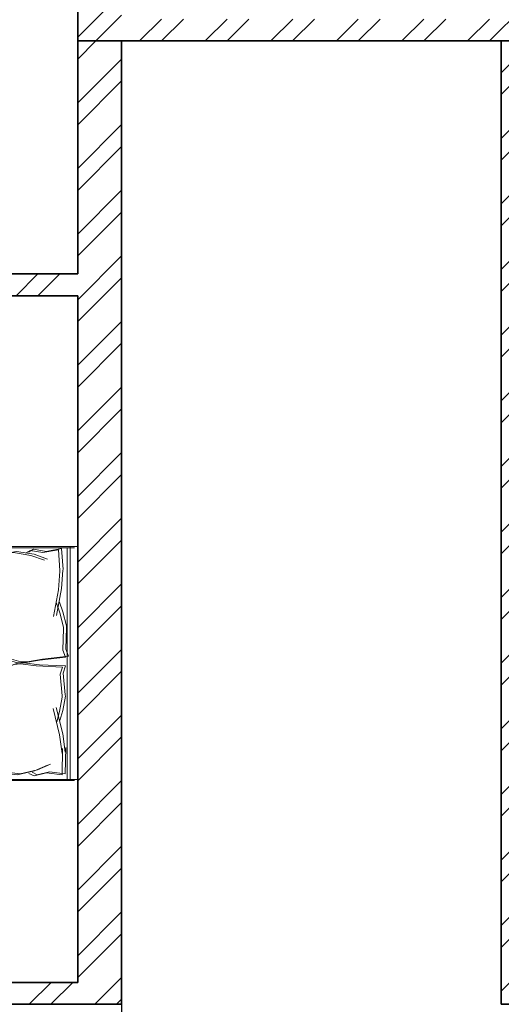
# Model space of a CAD drawing. Units: inches. Extents: x 2120 to 4013, y 1390 to 3019.
# Tile 13 of 59: x 2617 to 2716, y 1582 to 1784. Entities that reach past the tile are written whole.
import ezdxf

# ---------------------------------------------------------------- set-up
doc = ezdxf.new("R2010")
doc.units = ezdxf.units.IN
for name, color, linetype, lineweight in [('A-FLOR-DECK', 7, 'Continuous', 25), ('A-FURN', 8, 'Continuous', 13), ('A-WALL', 7, 'Continuous', 35), ('A-WALL-PATT', 252, 'Continuous', 13)]:
    doc.layers.add(name, color=color, linetype=linetype, lineweight=lineweight)

# ---------------------------------------------------------------- blocks, each defined once
blk = doc.blocks.new('BED-DOUBLE-PLAN')
for p, q in [((3.48, 63.34), (3.48, 81.45)), ((3.48, 81.45), (51.27, 81.45)), ((51.27, 81.45), (51.27, 54.84)), ((3.48, 79.91), (51.27, 79.91)), ((3.7, 62.7), (3.7, 80.81)), ((3.7, 79.27), (51.5, 79.27)), ((16.88, 78.42), (19.77, 79.14)), ((19.77, 79.14), (20.09, 79.14)), ((20.09, 79.14), (24.54, 79)), ((24.54, 79), (25.98, 79.58)), ((24.77, 78.36), (26.21, 78.94)), ((25.98, 79.58), (26.56, 74.23)), ((26.21, 78.94), (26.79, 73.59)), ((27.98, 78.95), (27.73, 73.58)), ((29.46, 78.47), (27.98, 78.95)), ((33.89, 78.89), (29.46, 78.47)), ((34.21, 78.91), (33.89, 78.89)), ((37.14, 78.37), (34.21, 78.91)), ((45.71, 78.9), (41.92, 78.38)), ((50.11, 78.89), (44.71, 78.99)), ((44.71, 78.99), (45.71, 78.9)), ((50.11, 78.89), (49.73, 75.68)), ((51.5, 80.81), (51.5, 54.2)), ((3.9, 78.11), (8.18, 78.44)), ((3.9, 78.13), (4.47, 74.95)), ((4.12, 77.49), (4.7, 74.31)), ((4.13, 77.47), (8.41, 77.8)), ((8.18, 78.44), (8.29, 78.42)), ((8.29, 78.42), (12.11, 78.13)), ((8.41, 77.8), (8.51, 77.78)), ((8.51, 77.78), (12.34, 77.49)), ((12.11, 78.13), (17.6, 77.12)), ((12.34, 77.49), (17.83, 76.48)), ((14.86, 77.7), (16.88, 78.42)), ((15.08, 77.06), (17.11, 77.78)), ((17.11, 77.78), (20, 78.5)), ((20, 78.5), (20.32, 78.5)), ((20.32, 78.5), (24.77, 78.36)), ((28.21, 78.32), (27.96, 72.94)), ((29.69, 77.83), (28.21, 78.32)), ((34.11, 78.25), (29.69, 77.83)), ((34.43, 78.27), (34.11, 78.25)), ((37.37, 77.73), (34.43, 78.27)), ((41.92, 78.38), (36.5, 77.02)), ((42.14, 77.74), (36.72, 76.38)), ((39.2, 77.77), (37.14, 78.37)), ((39.43, 77.13), (37.37, 77.73)), ((45.94, 78.26), (42.14, 77.74)), ((50.34, 78.25), (44.94, 78.35)), ((44.94, 78.35), (45.94, 78.26)), ((50.34, 78.25), (49.96, 75.04)), ((4.47, 74.95), (4.04, 72.35)), ((5.05, 72.49), (6.06, 75.24)), ((49.31, 73.19), (48.13, 75.87)), ((49.54, 72.55), (48.36, 75.23)), ((49.73, 75.68), (50.33, 73.11)), ((49.96, 75.04), (50.56, 72.47)), ((4.7, 74.31), (4.27, 71.71)), ((5.28, 71.85), (6.29, 74.6)), ((26.56, 74.23), (27.14, 71.05)), ((26.79, 73.59), (27.37, 70.41)), ((27.73, 73.58), (27.36, 70.37)), ((27.96, 72.94), (27.58, 69.73)), ((50.11, 69.62), (49.31, 73.19)), ((50.33, 73.11), (49.82, 72.06)), ((4.04, 72.35), (4.62, 71.33)), ((4.27, 71.71), (4.85, 70.7)), ((4.47, 68.88), (5.05, 72.49)), ((4.7, 68.24), (5.28, 71.85)), ((27.14, 71.05), (27.14, 69.74)), ((50.34, 68.98), (49.54, 72.55)), ((50.56, 72.47), (50.04, 71.42)), ((4.76, 67.29), (4.47, 68.88)), ((27.14, 69.74), (26.56, 67.86)), ((27.37, 69.1), (26.79, 67.23)), ((27.36, 70.37), (27.44, 69.07)), ((27.37, 70.41), (27.37, 69.1)), ((27.44, 69.07), (28.13, 67.23)), ((27.58, 69.73), (27.67, 68.43)), ((49.92, 68.01), (50.11, 69.62)), ((50.15, 67.37), (50.34, 68.98)), ((4.19, 64.11), (4.76, 67.29)), ((4.99, 66.65), (4.7, 68.24)), ((26.56, 67.86), (26.56, 65.18)), ((26.79, 67.23), (26.79, 64.54)), ((27.67, 68.43), (28.36, 66.59)), ((28.13, 67.23), (28.3, 64.55)), ((50.7, 64.87), (49.92, 68.01)), ((50.93, 64.23), (50.15, 67.37)), ((9.28, 64.83), (4.19, 64.11)), ((4.41, 63.47), (4.99, 66.65)), ((6.38, 65.82), (10.42, 65.15)), ((6.61, 65.18), (10.64, 64.51)), ((10.42, 65.15), (9.28, 64.83)), ((10.42, 65.15), (17.43, 64.72)), ((17.43, 64.72), (19.39, 65.28)), ((19.39, 65.28), (24.52, 64.87)), ((24.1, 65.18), (20.96, 66.27)), ((24.33, 64.54), (21.19, 65.63)), ((26.56, 65.18), (24.1, 65.18)), ((28.3, 64.55), (30.75, 64.71)), ((28.36, 66.59), (28.53, 63.91)), ((30.75, 64.71), (33.82, 65.99)), ((30.98, 64.07), (34.05, 65.35)), ((32.57, 65.82), (36.6, 65.15)), ((32.79, 65.18), (36.83, 64.51)), ((36.6, 65.15), (43.61, 64.72)), ((43.61, 64.72), (45.57, 65.28)), ((45.57, 65.28), (50.7, 64.87)), ((9.51, 64.19), (4.41, 63.47)), ((10.64, 64.51), (9.51, 64.19)), ((10.64, 64.51), (17.65, 64.08)), ((17.65, 64.08), (19.61, 64.64)), ((19.61, 64.64), (24.75, 64.23)), ((26.79, 64.54), (24.33, 64.54)), ((28.53, 63.91), (30.98, 64.07)), ((30.26, 64.06), (34.45, 57.57)), ((30.49, 63.42), (34.68, 56.93)), ((40.65, 61.13), (32.31, 64.06)), ((40.87, 60.49), (32.54, 63.42)), ((36.83, 64.51), (43.84, 64.08)), ((43.84, 64.08), (45.8, 64.64)), ((45.8, 64.64), (50.93, 64.23)), ((46.22, 59.12), (40.65, 61.13)), ((46.45, 58.48), (40.87, 60.49)), ((49.16, 56.95), (46.22, 59.12)), ((34.45, 57.57), (36.15, 53.08)), ((34.68, 56.93), (36.38, 52.44)), ((49.39, 56.31), (46.45, 58.48)), ((52.87, 53.7), (49.16, 56.95)), ((53.1, 53.06), (49.39, 56.31)), ((36.15, 53.08), (36.46, 51.07)), ((38.94, 51.69), (40.96, 52.62)), ((40.96, 52.62), (44.36, 53.08)), ((44.36, 53.08), (48.23, 53.39)), ((44.59, 52.44), (48.46, 52.75)), ((48.23, 53.39), (51.33, 53.08)), ((48.46, 52.75), (51.56, 52.44)), ((51.33, 53.08), (52.87, 53.7)), ((51.56, 52.44), (53.1, 53.06)), ((52.95, 51.96), (52.87, 53.7, 3.87)), ((53.18, 51.32), (53.1, 53.06, 3.87)), ((36.38, 52.44), (36.69, 50.43)), ((36.46, 51.07), (38.94, 51.69)), ((36.69, 50.43), (39.17, 51.05)), ((39.17, 51.05), (41.18, 51.98)), ((41.18, 51.98), (44.59, 52.44)), ((15.06, 2.2), (39.68, 2.2)), ((15.29, 1.56), (39.91, 1.56))]:
    blk.add_line(p, q)
for centre, radius, start, end in [((85.16, 61.35), 83.31, 178.7218, 185.604), ((21.36, -100.61), 164.97, 86.0865, 96.7821), ((21.59, -101.25), 164.97, 86.0865, 96.7821), ((85.39, 60.71), 83.31, 178.7218, 185.604), ((17.76, -74.87), 129.02, 81.7845, 96.9006), ((17.99, -75.51), 129.02, 81.7845, 96.9006), ((-167.31, 50.27), 170.11, 358.4762, 1.0082), ((-167.08, 49.63), 170.11, 358.4762, 1.0082), ((43.74, 46.38), 6.22, 78.6608, 113.7384), ((36.64, 51.01), 0.185, 160.2464, 271.1377), ((31.16, 79.96), 29.65, 280.6617, 289.8806), ((31.38, 79.32), 29.65, 280.6617, 289.8806), ((43.97, 45.74), 6.22, 78.6608, 113.7384), ((51.33, 88.1), 36.18, 259.8763, 272.5657), ((51.56, 87.46), 36.18, 259.8763, 272.5657), ((182.27, 45.13), 129.5, 176.9791, 183.8365), ((182.5, 44.49), 129.5, 176.9791, 183.8365), ((36.87, 50.37), 0.185, 160.2464, 271.1377), ((484.82, 30.83), 482.31, 178.2277, 181.7185), ((485.05, 30.19), 482.31, 178.2277, 181.7185), ((-4508.74, 13.62), 4561.86, 0.00217, 0.28689), ((-4508.51, 12.99), 4561.86, 0.00217, 0.28689), ((-26.9, 16.93), 29.63, 346.0648, 358.9113), ((-26.67, 16.29), 29.63, 346.0648, 358.9113), ((76.16, 12.78), 23.07, 177.4714, 206.4681), ((76.39, 12.14), 23.07, 177.4714, 206.4681), ((-21.66, 11.17), 23.56, 337.9751, 356.652), ((-21.43, 10.53), 23.56, 337.9751, 356.652), ((1.09, 1.73), 1.09, 146.1736, 293.4781), ((21.43, -119.39), 121.76, 92.9958, 99.4091), ((-17.22, 105.16), 106.46, 283.3832, 287.7053), ((-16.99, 104.52), 106.46, 283.3832, 287.7053), ((41.15, -130.83), 133.04, 84.4998, 90.6351), ((54.41, 2.58), 1.1, 242.6588, 356.02), ((1.32, 1.09), 1.09, 146.1736, 293.4781), ((21.66, -120.03), 121.76, 92.9958, 99.4091), ((41.38, -131.47), 133.04, 84.4998, 90.6351), ((54.64, 1.94), 1.1, 242.6588, 356.02)]:
    blk.add_arc(centre, radius, start, end)

msp = doc.modelspace()

# ---------------------------------------------------------------- hatches: boundary and pattern name
at = {"layer": 'A-WALL-PATT'}
h = msp.add_hatch(dxfattribs=at)
h.set_pattern_fill('ANSI32', color=256)
h.paths.add_polyline_path([(2271.7331, 2122.6377), (2262.7331, 2122.6377), (2262.7331, 2040.3893), (2267.2331, 2040.3893), (2271.7331, 2040.3893), (2271.7331, 2044.8856), (2271.7331, 2070.531), (2391.7331, 2070.531), (2391.7331, 1926.5306), (2388.3993, 1926.5306), (2388.3993, 1922.531), (2395.7331, 1922.531), (2395.7331, 1992.531), (2400.4511, 1992.531), (2400.4511, 1997.0306), (2395.7331, 1997.0306), (2395.7331, 2070.531), (2443.7331, 2070.531), (2443.7331, 2046.1368), (2448.2331, 2046.1368), (2448.2331, 2070.531), (2580.2331, 2070.531), (2580.2331, 1997.0306), (2492.9076, 1997.0306), (2492.9076, 1992.531), (2580.2331, 1992.531), (2580.2331, 1983.9368), (2589.2331, 1983.9368), (2589.2331, 2070.531), (2589.2331, 2075.0306), (2396.2331, 2075.0306), (2396.2331, 2184.3565), (2393.9831, 2184.3565), (2391.7331, 2184.3565), (2391.7331, 2075.0306), (2271.7331, 2075.0306)])
h.paths.add_polyline_path([(2724.7331, 2138.0306), (2628.7331, 2138.0306), (2628.7331, 2070.5306), (2628.7331, 2067.0987), (2633.2331, 2067.0987), (2637.7331, 2067.0987), (2637.7331, 2070.531), (2657.3413, 2070.531), (2657.3413, 2079.5306), (2637.7331, 2079.5306), (2637.7331, 2129.031), (2715.7331, 2129.031), (2715.7331, 2079.5306), (2698.0378, 2079.5306), (2698.0378, 2070.531), (2715.7331, 2070.531), (2715.7331, 2012.1531), (2720.2331, 2012.1531), (2724.7331, 2012.1531)])
h.paths.add_polyline_path([(2724.7331, 2213.031), (2831.3209, 2213.031), (2831.3209, 2215.281), (2831.3209, 2217.5306), (2724.7331, 2217.5306), (2724.7331, 2343.531), (2751.8755, 2343.531), (2751.8755, 2352.5306), (2715.7331, 2352.5306), (2715.7331, 2138.031), (2724.7331, 2138.031)])
h.paths.add_polyline_path([(2902.53, 2352.5306), (2811.8755, 2352.5306), (2811.8755, 2343.531), (2867.2331, 2343.531), (2867.2331, 2217.5306), (2863.6364, 2217.5306), (2863.6364, 2213.031), (2871.7331, 2213.031), (2871.7331, 2217.531), (2871.7331, 2343.531), (2902.53, 2343.531)])
h.paths.add_polyline_path([(3009.7331, 2352.5306), (2938.53, 2352.5306), (2938.53, 2343.531), (2966.2331, 2343.531), (2966.2331, 2242.3281), (2968.4831, 2242.3281), (2970.7331, 2242.3281), (2970.7331, 2343.531), (3009.7331, 2343.531)])
h.paths.add_polyline_path([(3009.7331, 2217.5306), (2970.7331, 2217.5306), (2970.7331, 2220.5422), (2968.4831, 2220.5422), (2966.2331, 2220.5422), (2966.2331, 2217.5306), (2911.7752, 2217.5306), (2907.7331, 2217.5306), (2907.7331, 2213.0306), (2907.7331, 2194.9663), (2912.2331, 2194.9663), (2912.2331, 2213.031), (2970.7331, 2213.031), (3000.7331, 2213.031), (3000.7331, 2205.523), (3009.7331, 2205.523)])
h.paths.add_polyline_path([(3009.7331, 2181.5227), (3000.7331, 2181.5227), (3000.7331, 2165.0306), (2912.2331, 2165.0306), (2912.2331, 2170.8202), (2907.7331, 2170.8202), (2907.7331, 2165.0306), (2899.5169, 2165.0306), (2899.5169, 2162.7806), (2899.5169, 2160.531), (2907.7331, 2160.531), (2907.7331, 2137.3432), (2912.2331, 2137.3432), (2912.2331, 2160.531), (3000.7331, 2160.531), (3000.7331, 2150.4993), (3009.7331, 2150.4993)])
h.paths.add_polyline_path([(3009.7331, 2126.499), (3005.2331, 2126.499), (3000.7331, 2126.499), (3000.7331, 2112.5306), (2912.2331, 2112.5306), (2912.2331, 2115.6036), (2907.7331, 2115.6036), (2907.7331, 2108.031), (3000.7331, 2108.031), (3000.7331, 2084.7256), (3009.7331, 2084.7256)], flags=17)
h.paths.add_polyline_path([(3009.7331, 1971.531), (3009.7331, 2024.7253), (3000.7331, 2024.7253), (3000.7331, 2006.4153), (3000.7331, 1971.5306), (2864.2331, 1971.5306), (2864.2331, 2160.531), (2868.0522, 2160.531), (2868.0522, 2165.0306), (2859.7331, 2165.0306), (2859.7331, 1971.5306), (2724.7331, 1971.5306), (2724.7331, 1977.7012), (2715.7331, 1977.7012), (2715.7331, 1962.5306), (2715.7331, 1950.9035), (2720.2331, 1950.9035), (2724.7331, 1950.9035), (2724.7331, 1962.531), (2855.2331, 1962.531), (2859.7331, 1962.531), (2859.7331, 1835.031), (2864.2331, 1834.8158), (2864.2331, 1962.531), (2958.7331, 1962.531), (2958.7331, 1937.0925), (2963.2331, 1937.0925), (2963.2331, 1962.531), (3000.7331, 1962.531), (3009.7331, 1962.531)])
h.paths.add_polyline_path([(2724.7331, 1728.531), (2822.7164, 1728.531), (2822.7164, 1733.0306), (2724.7331, 1733.0306), (2724.7331, 1779.3416), (2715.7331, 1779.3416), (2715.7331, 1581.531), (2753.02, 1581.531), (2753.02, 1586.031), (2753.02, 1590.5306), (2724.7331, 1590.5306)])
h.paths.add_polyline_path([(2864.2331, 1590.531), (2864.2331, 1787.031), (2868.4075, 1787.031), (2868.4075, 1791.5306), (2859.7331, 1791.5306), (2859.7331, 1739.0306), (2859.7331, 1733.0306), (2854.3125, 1733.0306), (2854.3125, 1728.531), (2859.7331, 1728.531), (2859.7331, 1590.5306), (2813.02, 1590.5306), (2813.02, 1581.531), (2868.4123, 1581.531), (2868.4123, 1583.781), (2868.4123, 1586.0306), (2864.2331, 1586.0306)])
h.paths.add_polyline_path([(3009.7331, 1754.6619), (3000.7331, 1754.6619), (3000.7331, 1739.0306), (2912.2331, 1739.0306), (2912.2331, 1742.2257), (2907.7331, 1742.2257), (2907.7331, 1739.0306), (2907.7331, 1734.531), (3000.7331, 1734.531), (3000.7331, 1590.5306), (3000.7331, 1586.0306), (2971.3921, 1586.0306), (2971.3921, 1581.531), (3009.7331, 1581.531)])
h.paths.add_polyline_path([(2911.3921, 1583.781), (2911.3921, 1586.0306), (2891.2138, 1586.0306), (2891.2138, 1581.531), (2911.3921, 1581.531)])
h.paths.add_polyline_path([(3009.7331, 1799.8422), (3000.7331, 1799.8422), (3000.7331, 1791.5306), (2912.2331, 1791.5306), (2912.2331, 1796.3264), (2909.9831, 1796.3264), (2907.7331, 1796.3264), (2907.7331, 1791.5306), (2902.7033, 1791.5306), (2902.7033, 1787.031), (2907.7331, 1787.031), (2907.7331, 1761.1622), (2912.2331, 1761.1622), (2912.2331, 1787.031), (3000.7331, 1787.031), (3000.7331, 1778.6622), (3009.7331, 1778.6622)])
h.paths.add_polyline_path([(3009.7331, 1839.5306), (2963.2331, 1839.5306), (2963.2331, 1842.8629), (2960.9831, 1842.8629), (2958.7331, 1842.8629), (2958.7331, 1839.5306), (2907.7331, 1839.5306), (2907.7331, 1814.4599), (2912.2331, 1814.4599), (2912.2331, 1835.031), (3000.7331, 1835.031), (3000.7331, 1823.8425), (3009.7331, 1823.8425), (3009.7331, 1835.031)])
h.paths.add_polyline_path([(2963.2331, 1901.0922), (2960.9831, 1901.0922), (2958.7331, 1901.0922), (2958.7331, 1862.8843), (2963.2331, 1862.8843)], flags=17)
h.paths.add_polyline_path([(2724.7331, 1891.9826), (2724.7331, 1914.3416), (2715.7331, 1914.3416), (2715.7331, 1783.8416), (2637.7331, 1783.8416), (2637.7331, 1914.3416), (2628.7331, 1914.3416), (2624.7701, 1914.3416), (2624.7701, 1909.8416), (2624.7701, 1905.3419), (2628.7331, 1905.3419), (2628.7331, 1876.9915), (2628.7331, 1779.3419), (2637.7331, 1779.3419), (2715.7331, 1779.3419), (2724.7331, 1779.3419), (2724.7331, 1835.031)])
h.paths.add_polyline_path([(2637.7331, 1731.531), (2637.7331, 1779.3416), (2628.7331, 1779.3416), (2628.7331, 1731.5306), (2589.2331, 1731.5306), (2535.9814, 1731.5306), (2496.7331, 1731.5306), (2496.7331, 1725.6876), (2498.9831, 1725.6876), (2501.2331, 1725.6876), (2501.2331, 1727.031), (2628.7331, 1727.031), (2628.7331, 1680.4203), (2628.7331, 1590.5306), (2628.7331, 1586.0306), (2604.1361, 1586.0306), (2604.1361, 1581.531), (2637.7331, 1581.531), (2637.7331, 1590.531)])

# ---------------------------------------------------------------- linework, layer by layer
at = {"layer": 'A-FLOR-DECK'}
msp.add_line((2637.7331, 1581.531), (2637.7331, 1542.531), dxfattribs=at)
at = {"layer": 'A-WALL'}
for p, q in [((2628.7331, 1731.531), (2628.7331, 1876.9918)), ((2628.7331, 1731.5306), (2628.7331, 1876.9915)), ((2637.7331, 1779.3419), (2628.7331, 1779.3419)), ((2637.7331, 1779.3416), (2628.7331, 1779.3416)), ((2715.7331, 1779.3419), (2637.7331, 1779.3419)), ((2637.7331, 1779.3419), (2637.7331, 1680.4206)), ((2637.7331, 1779.3416), (2637.7331, 1680.4203)), ((2715.7331, 1779.3416), (2637.7331, 1779.3416)), ((2715.7331, 1779.3419), (2724.7331, 1779.3419)), ((2715.7331, 1779.3419), (2715.7331, 1581.531)), ((2715.7331, 1779.3416), (2715.7331, 1581.5306)), ((2715.7331, 1779.3416), (2724.7331, 1779.3416)), ((2589.2331, 1731.531), (2628.7331, 1731.531)), ((2589.2331, 1731.5306), (2628.7331, 1731.5306)), ((2637.7331, 1731.531), (2637.7331, 1590.531)), ((2637.7331, 1731.5306), (2637.7331, 1590.5306)), ((2501.2331, 1727.031), (2628.7331, 1727.031)), ((2501.2331, 1727.0306), (2628.7331, 1727.0306)), ((2628.7331, 1680.4206), (2628.7331, 1727.031)), ((2628.7331, 1680.4203), (2628.7331, 1727.0306)), ((2628.7331, 1680.4206), (2628.7331, 1590.531)), ((2628.7331, 1680.4203), (2628.7331, 1590.5306)), ((2628.7331, 1586.031), (2628.7331, 1590.531)), ((2628.7331, 1586.0306), (2628.7331, 1590.5306)), ((2637.7331, 1590.531), (2637.7331, 1581.531)), ((2637.7331, 1590.5306), (2637.7331, 1581.5306)), ((2527.1368, 1586.031), (2628.7331, 1586.031)), ((2527.1368, 1586.0306), (2628.7331, 1586.0306)), ((2637.7331, 1581.531), (2525.3594, 1581.531)), ((2870.4123, 1581.531), (2715.7331, 1581.531))]:
    msp.add_line(p, q, dxfattribs=at)

# ---------------------------------------------------------------- block references
at = {"layer": 'A-FURN', "rotation": 270}
for p in [(2547.2869, 1678.9956), (2547.2869, 1678.9953)]:
    msp.add_blockref('BED-DOUBLE-PLAN', p, dxfattribs=at)

doc.saveas('drawing.dxf')
